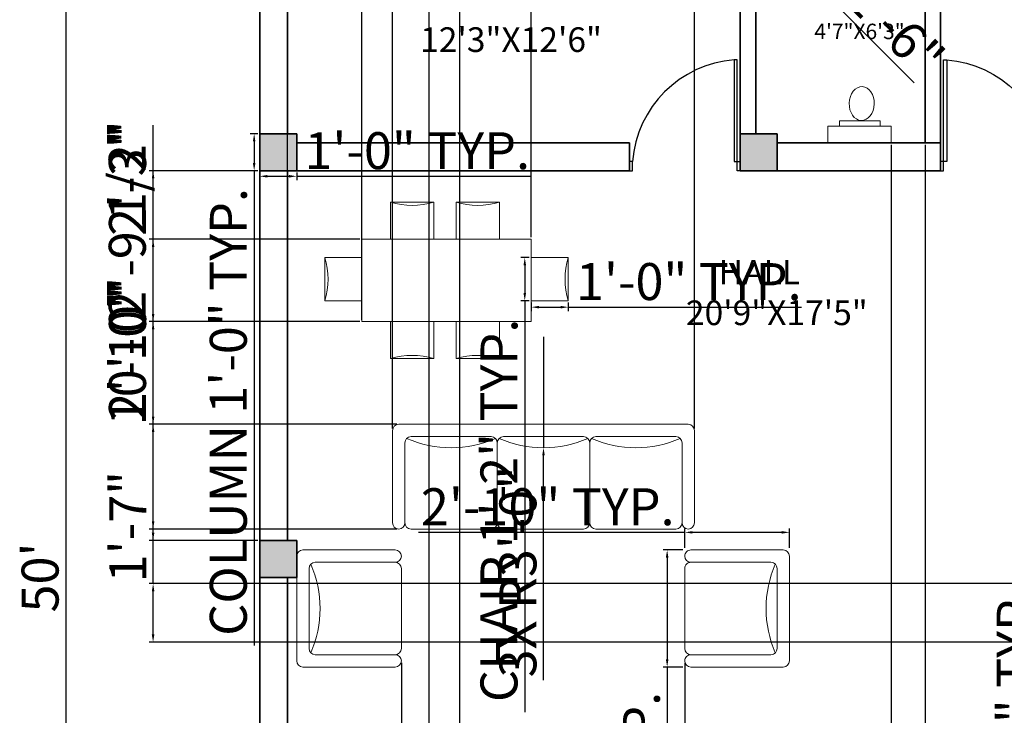
# Model space of a CAD drawing. Units: inches. Extents: x 2430 to 3058, y 1630 to 2396.
# Tile 2 of 4: x 2558 to 2878, y 1945 to 2171. Entities that reach past the tile are written whole.
import ezdxf

# ---------------------------------------------------------------- set-up
doc = ezdxf.new("R2010")
doc.units = ezdxf.units.IN
for name, color, linetype, lineweight in [('A-ANNO-DIMS', 7, 'Continuous', 18), ('A-AREA-IDEN', 131, 'Continuous', 18), ('A-COLS', 7, 'Continuous', 35), ('A-COLS-PATT', 1, 'Continuous', 13), ('A-DOOR', 40, 'Continuous', 25), ('A-FLOR-FIXT', 2, 'Continuous', 18), ('A-WALL', 7, 'Continuous', 35)]:
    doc.layers.add(name, color=color, linetype=linetype, lineweight=lineweight)
doc.layers.add('A-FURN', color=33, linetype='Continuous', lineweight=18, true_color=0xb0a07d)
doc.styles.get("Standard").update_dxf_attribs({"font": 'arial.ttf'})
doc.dimstyles.new('ISO-25', dxfattribs={"dimtxt": 12, "dimasz": 2.5, "dimexe": 1.25, "dimexo": 0.625, "dimtad": 1, "dimdec": 0, "dimlunit": 3, "dimtxsty": 'Standard', "dimcen": 2.5, "dimadec": 0, "dimazin": 0, "dimtfac": 1, "dimtdec": 0, "dimtmove": 0, "dimatfit": 3, "dimfxl": 1, "dimarcsym": 0})

# ---------------------------------------------------------------- blocks, each defined once
blk = doc.blocks.new('*D2')
at = {"layer": 'A-ANNO-DIMS', "color": 0, "lineweight": -2, "transparency": 16777216}
for p, q in [((2635.37, 2289.88), (2571.77, 2289.88)), ((2573.02, 2287.38), (2573.02, 1692.38)), ((2635.37, 1689.88), (2571.77, 1689.88))]:
    blk.add_line(p, q, dxfattribs=at)
at = {"layer": 'A-ANNO-DIMS', "color": 0, "transparency": 16777216}
for points in [[(2572.61, 2287.38), (2573.44, 2287.38), (2573.02, 2289.88)], [(2572.61, 1692.38), (2573.44, 1692.38), (2573.02, 1689.88)]]:
    blk.add_solid(points, dxfattribs=at)
at = {"layer": 'Defpoints', "color": 0, "transparency": 16777216}
for p in [(2636, 2289.88), (2573.02, 1689.88), (2636, 1689.88)]:
    blk.add_point(p, dxfattribs=at)
at = {"layer": 'A-ANNO-DIMS', "color": 0, "transparency": 16777216, "insert": (2566.27, 1989.88), "char_height": 12, "attachment_point": 5, "rotation": 90}
blk.add_mtext("50'", dxfattribs=at)
blk = doc.blocks.new('WC')
for points in [[(0, 18.29), (20.63, 18.29), (20.63, 12.83), (0, 12.83)], [(3.58, 12.83), (16.78, 12.83), (16.78, 11.1), (3.58, 11.1)]]:
    blk.add_lwpolyline(points, close=True)
blk.add_ellipse((9.59, 5.49), major_axis=(0.18, 5.49), ratio=0.738535)
blk = doc.blocks.new('ARMCHAIR')
for p, q in [((0, 2), (0, 36)), ((2, 38), (32, 38)), ((34, 36), (34, 36)), ((4, 6), (4, 32)), ((6, 34), (32, 34)), ((34, 32), (34, 6)), ((32, 4), (6, 4)), ((32, 0), (2, 0)), ((34, 2), (34, 2))]:
    blk.add_line(p, q)
for centre, radius, start, end in [((2, 36), 2, 90, 180), ((32, 36), 2, 0, 90), ((32, 36), 2, 270, 0), ((6, 32), 2, 90, 180), ((-28.4, 19), 36, 336.3971, 23.6029), ((32, 32), 2, 0, 90), ((6, 6), 2, 180, 270), ((32, 6), 2, 270, 0), ((32, 2), 2, 0, 90), ((2, 2), 2, 180, 270), ((32, 2), 2, 270, 0)]:
    blk.add_arc(centre, radius, start, end)
blk = doc.blocks.new('DOOR-36')
for p, q in [((35, 36), (34, 36)), ((34, 36), (34, 3)), ((35, 0), (35, 36)), ((1, 3), (0, 3)), ((0, 0), (1, 0)), ((1, 0), (1, 3)), ((34, 3), (36, 3)), ((36, 0), (35, 0))]:
    blk.add_line(p, q)
blk.add_arc((36.88, 0.12), 36, 94.5954, 175.4046)
blk = doc.blocks.new('CHAIR-DINING')
for p, q in [((0, 0), (0, 12)), ((0, 12), (14, 12)), ((14, 12), (14, 0))]:
    blk.add_line(p, q)
blk.add_arc((7, 34.96), 24, 253.0422, 286.9578)
blk = doc.blocks.new('COL-12x12-EDGE')
for p, q in [((12, 12), (0, 12)), ((0, 12), (0, 0)), ((0, 0), (12, 0))]:
    blk.add_line(p, q)
blk = doc.blocks.new('COL-12x12')
for p, q in [((12, 12), (0, 12)), ((0, 12), (0, 0)), ((12, 0), (12, 12)), ((0, 0), (12, 0))]:
    blk.add_line(p, q)
blk = doc.blocks.new('*D13')
at = {"layer": 'A-ANNO-DIMS', "color": 0, "lineweight": -2, "transparency": 16777216}
for p, q in [((2635.37, 2133.88), (2632.95, 2133.88)), ((2634.2, 2131.38), (2634.2, 2124.38)), ((2635.37, 2121.88), (2632.95, 2121.88)), ((2634.2, 2121.88), (2634.2, 1967.82))]:
    blk.add_line(p, q, dxfattribs=at)
at = {"layer": 'A-ANNO-DIMS', "color": 0, "transparency": 16777216}
for points in [[(2633.78, 2131.38), (2634.61, 2131.38), (2634.2, 2133.88)], [(2633.78, 2124.38), (2634.61, 2124.38), (2634.2, 2121.88)]]:
    blk.add_solid(points, dxfattribs=at)
at = {"layer": 'Defpoints', "color": 0, "transparency": 16777216}
for p in [(2636, 2133.88), (2634.2, 2121.88), (2636, 2121.88)]:
    blk.add_point(p, dxfattribs=at)
at = {"layer": 'A-ANNO-DIMS', "color": 0, "transparency": 16777216, "insert": (2627.36, 2043.6), "char_height": 12, "attachment_point": 5, "rotation": 90}
blk.add_mtext('COLUMN 1\'-0" TYP.', dxfattribs=at)
blk = doc.blocks.new('*D14')
at = {"layer": 'A-ANNO-DIMS', "color": 0, "lineweight": -2, "transparency": 16777216}
for p, q in [((2636, 2121.25), (2636, 2118.83)), ((2638.5, 2120.08), (2645.5, 2120.08)), ((2648, 2121.25), (2648, 2118.83)), ((2648, 2120.08), (2723.76, 2120.08))]:
    blk.add_line(p, q, dxfattribs=at)
at = {"layer": 'A-ANNO-DIMS', "color": 0, "transparency": 16777216}
for points in [[(2638.5, 2120.49), (2638.5, 2119.66), (2636, 2120.08)], [(2645.5, 2120.49), (2645.5, 2119.66), (2648, 2120.08)]]:
    blk.add_solid(points, dxfattribs=at)
at = {"layer": 'Defpoints', "color": 0, "transparency": 16777216}
for p in [(2636, 2121.88), (2648, 2121.88), (2648, 2120.08)]:
    blk.add_point(p, dxfattribs=at)
at = {"layer": 'A-ANNO-DIMS', "color": 0, "transparency": 16777216, "insert": (2687.13, 2126.83), "char_height": 12, "attachment_point": 5}
blk.add_mtext('1\'-0" TYP.', dxfattribs=at)
blk = doc.blocks.new('*D19')
at = {"layer": 'A-ANNO-DIMS', "color": 0, "lineweight": -2, "transparency": 16777216}
for p, q in [((2894.37, 2028.88), (2888.35, 2028.88)), ((2889.6, 2026.38), (2889.6, 1995.38)), ((2894.37, 1992.88), (2888.35, 1992.88)), ((2889.6, 1992.88), (2889.6, 1861.63))]:
    blk.add_line(p, q, dxfattribs=at)
at = {"layer": 'A-ANNO-DIMS', "color": 0, "transparency": 16777216}
for points in [[(2889.18, 2026.38), (2890.01, 2026.38), (2889.6, 2028.88)], [(2889.18, 1995.38), (2890.01, 1995.38), (2889.6, 1992.88)]]:
    blk.add_solid(points, dxfattribs=at)
at = {"layer": 'Defpoints', "color": 0, "transparency": 16777216}
for p in [(2895, 2028.88), (2889.6, 1992.88), (2895, 1992.88)]:
    blk.add_point(p, dxfattribs=at)
at = {"layer": 'A-ANNO-DIMS', "color": 0, "transparency": 16777216, "insert": (2882.76, 1926), "char_height": 12, "attachment_point": 5, "rotation": 90}
blk.add_mtext('DOOR 3\'-0" TYP.', dxfattribs=at)
blk = doc.blocks.new('*D23')
at = {"layer": 'A-ANNO-DIMS', "color": 0, "lineweight": -2, "transparency": 16777216}
for p, q in [((2723.51, 2093.7), (2720.79, 2093.7)), ((2722.04, 2091.2), (2722.04, 2082.2)), ((2723.51, 2079.7), (2720.79, 2079.7)), ((2722.04, 2079.7), (2722.04, 1946.13))]:
    blk.add_line(p, q, dxfattribs=at)
at = {"layer": 'A-ANNO-DIMS', "color": 0, "transparency": 16777216}
for points in [[(2721.62, 2091.2), (2722.45, 2091.2), (2722.04, 2093.7)], [(2721.62, 2082.2), (2722.45, 2082.2), (2722.04, 2079.7)]]:
    blk.add_solid(points, dxfattribs=at)
at = {"layer": 'Defpoints', "color": 0, "transparency": 16777216}
for p in [(2724.14, 2093.7), (2722.04, 2079.7), (2724.14, 2079.7)]:
    blk.add_point(p, dxfattribs=at)
at = {"layer": 'A-ANNO-DIMS', "color": 0, "transparency": 16777216, "insert": (2715.21, 2011.66), "char_height": 12, "attachment_point": 5, "rotation": 90}
blk.add_mtext('CHAIR 1\'-2" TYP.', dxfattribs=at)
blk = doc.blocks.new('*D24')
at = {"layer": 'A-ANNO-DIMS', "color": 0, "lineweight": -2, "transparency": 16777216}
for p, q in [((2724.14, 2079.08), (2724.14, 2076.35)), ((2726.64, 2077.6), (2733.64, 2077.6)), ((2736.14, 2079.08), (2736.14, 2076.35)), ((2736.14, 2077.6), (2811.9, 2077.6))]:
    blk.add_line(p, q, dxfattribs=at)
at = {"layer": 'A-ANNO-DIMS', "color": 0, "transparency": 16777216}
for points in [[(2726.64, 2078.02), (2726.64, 2077.18), (2724.14, 2077.6)], [(2733.64, 2078.02), (2733.64, 2077.18), (2736.14, 2077.6)]]:
    blk.add_solid(points, dxfattribs=at)
at = {"layer": 'Defpoints', "color": 0, "transparency": 16777216}
for p in [(2724.14, 2079.7), (2736.14, 2079.7), (2736.14, 2077.6)]:
    blk.add_point(p, dxfattribs=at)
at = {"layer": 'A-ANNO-DIMS', "color": 0, "transparency": 16777216, "insert": (2775.27, 2084.35), "char_height": 12, "attachment_point": 5}
blk.add_mtext('1\'-0" TYP.', dxfattribs=at)
blk = doc.blocks.new('*D25')
at = {"layer": 'A-ANNO-DIMS', "color": 0, "lineweight": -2, "transparency": 16777216}
for p, q in [((2773.33, 1998.82), (2767, 1998.82)), ((2768.25, 1996.32), (2768.25, 1963.32)), ((2773.33, 1960.82), (2767, 1960.82)), ((2768.25, 1960.82), (2768.25, 1789.16))]:
    blk.add_line(p, q, dxfattribs=at)
at = {"layer": 'A-ANNO-DIMS', "color": 0, "transparency": 16777216}
for points in [[(2767.83, 1996.32), (2768.67, 1996.32), (2768.25, 1998.82)], [(2767.83, 1963.32), (2768.67, 1963.32), (2768.25, 1960.82)]]:
    blk.add_solid(points, dxfattribs=at)
at = {"layer": 'Defpoints', "color": 0, "transparency": 16777216}
for p in [(2773.95, 1998.82), (2768.25, 1960.82), (2773.95, 1960.82)]:
    blk.add_point(p, dxfattribs=at)
at = {"layer": 'A-ANNO-DIMS', "color": 0, "transparency": 16777216, "insert": (2761.42, 1873.74), "char_height": 12, "attachment_point": 5, "rotation": 90}
blk.add_mtext('ARMCHAIR 3\'-2" TYP.', dxfattribs=at)
blk = doc.blocks.new('*D26')
at = {"layer": 'A-ANNO-DIMS', "color": 0, "lineweight": -2, "transparency": 16777216}
for p, q in [((2773.95, 2004.52), (2687.53, 2004.52)), ((2773.95, 1999.45), (2773.95, 2005.77)), ((2805.45, 2004.52), (2776.45, 2004.52)), ((2807.95, 1999.45), (2807.95, 2005.77))]:
    blk.add_line(p, q, dxfattribs=at)
at = {"layer": 'A-ANNO-DIMS', "color": 0, "transparency": 16777216}
for points in [[(2776.45, 2004.94), (2776.45, 2004.11), (2773.95, 2004.52)], [(2805.45, 2004.94), (2805.45, 2004.11), (2807.95, 2004.52)]]:
    blk.add_solid(points, dxfattribs=at)
at = {"layer": 'Defpoints', "color": 0, "transparency": 16777216}
for p in [(2773.95, 2004.52), (2773.95, 1998.82), (2807.95, 1998.82)]:
    blk.add_point(p, dxfattribs=at)
at = {"layer": 'A-ANNO-DIMS', "color": 0, "transparency": 16777216, "insert": (2729.49, 2011.28), "char_height": 12, "attachment_point": 5}
blk.add_mtext('2\'-10" TYP.', dxfattribs=at)
blk = doc.blocks.new('*D44')
at = {"layer": 'A-ANNO-DIMS', "color": 0, "lineweight": -2, "transparency": 16777216}
for p, q in [((2691, 1913.5), (2691, 2325.73)), ((2693.5, 2324.48), (2698.5, 2324.48)), ((2701, 1913.5), (2701, 2325.73)), ((2701, 2324.48), (2745.97, 2324.48))]:
    blk.add_line(p, q, dxfattribs=at)
at = {"layer": 'A-ANNO-DIMS', "color": 0, "transparency": 16777216}
for points in [[(2693.5, 2324.89), (2693.5, 2324.06), (2691, 2324.48)], [(2698.5, 2324.89), (2698.5, 2324.06), (2701, 2324.48)]]:
    blk.add_solid(points, dxfattribs=at)
at = {"layer": 'Defpoints', "color": 0, "transparency": 16777216}
for p in [(2701, 2324.48), (2691, 1912.88), (2701, 1912.88)]:
    blk.add_point(p, dxfattribs=at)
at = {"layer": 'A-ANNO-DIMS', "color": 0, "transparency": 16777216, "insert": (2724.73, 2331.23), "char_height": 12, "attachment_point": 5}
blk.add_mtext('0\'-10"', dxfattribs=at)
blk = doc.blocks.new('*D49')
at = {"layer": 'A-ANNO-DIMS', "color": 0, "lineweight": -2, "transparency": 16777216}
for p, q in [((2840.99, 2130.25), (2840.99, 1630.03)), ((2852, 2130.25), (2852, 1630.03)), ((2843.49, 1631.28), (2849.5, 1631.28)), ((2852, 1631.28), (2896.97, 1631.28))]:
    blk.add_line(p, q, dxfattribs=at)
at = {"layer": 'A-ANNO-DIMS', "color": 0, "transparency": 16777216}
for points in [[(2843.49, 1631.69), (2843.49, 1630.86), (2840.99, 1631.28)], [(2849.5, 1631.69), (2849.5, 1630.86), (2852, 1631.28)]]:
    blk.add_solid(points, dxfattribs=at)
at = {"layer": 'Defpoints', "color": 0, "transparency": 16777216}
for p in [(2840.99, 2130.88), (2852, 2130.88), (2852, 1631.28)]:
    blk.add_point(p, dxfattribs=at)
at = {"layer": 'A-ANNO-DIMS', "color": 0, "transparency": 16777216, "insert": (2875.73, 1638.03), "char_height": 12, "attachment_point": 5}
blk.add_mtext('0\'-11"', dxfattribs=at)
blk = doc.blocks.new('*D51')
at = {"layer": 'A-ANNO-DIMS', "color": 0, "lineweight": -2, "transparency": 16777216}
for p, q in [((2601.4, 1987.88), (2601.4, 2022.4)), ((2899.37, 1987.88), (2600.15, 1987.88)), ((2601.4, 1971.38), (2601.4, 1985.38)), ((2899.37, 1968.88), (2600.15, 1968.88))]:
    blk.add_line(p, q, dxfattribs=at)
at = {"layer": 'A-ANNO-DIMS', "color": 0, "transparency": 16777216}
for points in [[(2600.98, 1985.38), (2601.81, 1985.38), (2601.4, 1987.88)], [(2600.98, 1971.38), (2601.81, 1971.38), (2601.4, 1968.88)]]:
    blk.add_solid(points, dxfattribs=at)
at = {"layer": 'Defpoints', "color": 0, "transparency": 16777216}
for p in [(2601.4, 1987.88), (2900, 1987.88), (2900, 1968.88)]:
    blk.add_point(p, dxfattribs=at)
at = {"layer": 'A-ANNO-DIMS', "color": 0, "transparency": 16777216, "insert": (2594.75, 2006.39), "char_height": 12, "attachment_point": 5, "rotation": 90}
blk.add_mtext('1\'-7"', dxfattribs=at)
blk = doc.blocks.new('*D58')
at = {"layer": 'A-ANNO-DIMS', "color": 0, "lineweight": -2, "transparency": 16777216}
for p, q in [((2669.13, 2100.28), (2669.13, 2325.73)), ((2671.63, 2324.48), (2721.64, 2324.48)), ((2724.14, 2100.28), (2724.14, 2325.73))]:
    blk.add_line(p, q, dxfattribs=at)
at = {"layer": 'A-ANNO-DIMS', "color": 0, "transparency": 16777216}
for points in [[(2671.63, 2324.89), (2671.63, 2324.06), (2669.13, 2324.48)], [(2721.64, 2324.89), (2721.64, 2324.06), (2724.14, 2324.48)]]:
    blk.add_solid(points, dxfattribs=at)
at = {"layer": 'Defpoints', "color": 0, "transparency": 16777216}
for p in [(2724.14, 2324.48), (2669.13, 2099.65), (2724.14, 2099.65)]:
    blk.add_point(p, dxfattribs=at)
at = {"layer": 'A-ANNO-DIMS', "color": 0, "transparency": 16777216, "insert": (2696.63, 2331.1), "char_height": 12, "attachment_point": 5}
blk.add_mtext('4\'-7"', dxfattribs=at)
blk = doc.blocks.new('*D59')
at = {"layer": 'A-ANNO-DIMS', "color": 0, "lineweight": -2, "transparency": 16777216}
for p, q in [((2601.4, 2099.65), (2601.4, 2135.51)), ((2668.5, 2099.65), (2600.15, 2099.65)), ((2601.4, 2075.4), (2601.4, 2097.15)), ((2668.5, 2072.9), (2600.15, 2072.9))]:
    blk.add_line(p, q, dxfattribs=at)
at = {"layer": 'A-ANNO-DIMS', "color": 0, "transparency": 16777216}
for points in [[(2600.98, 2097.15), (2601.81, 2097.15), (2601.4, 2099.65)], [(2600.98, 2075.4), (2601.81, 2075.4), (2601.4, 2072.9)]]:
    blk.add_solid(points, dxfattribs=at)
at = {"layer": 'Defpoints', "color": 0, "transparency": 16777216}
for p in [(2601.4, 2099.65), (2669.13, 2099.65), (2669.13, 2072.9)]:
    blk.add_point(p, dxfattribs=at)
at = {"layer": 'A-ANNO-DIMS', "color": 0, "transparency": 16777216, "insert": (2594.64, 2118.83), "char_height": 12, "attachment_point": 5, "rotation": 90}
blk.add_mtext('2\'-3"', dxfattribs=at)
blk = doc.blocks.new('*D60')
at = {"layer": 'A-ANNO-DIMS', "color": 0, "lineweight": -2, "transparency": 16777216}
for p, q in [((2679.11, 2038.23), (2679.11, 2325.73)), ((2681.61, 2324.48), (2774.61, 2324.48)), ((2777.11, 2038.23), (2777.11, 2325.73))]:
    blk.add_line(p, q, dxfattribs=at)
at = {"layer": 'A-ANNO-DIMS', "color": 0, "transparency": 16777216}
for points in [[(2681.61, 2324.89), (2681.61, 2324.06), (2679.11, 2324.48)], [(2774.61, 2324.89), (2774.61, 2324.06), (2777.11, 2324.48)]]:
    blk.add_solid(points, dxfattribs=at)
at = {"layer": 'Defpoints', "color": 0, "transparency": 16777216}
for p in [(2777.11, 2324.48), (2679.11, 2037.6), (2777.11, 2037.6)]:
    blk.add_point(p, dxfattribs=at)
at = {"layer": 'A-ANNO-DIMS', "color": 0, "transparency": 16777216, "insert": (2728.11, 2331.23), "char_height": 12, "attachment_point": 5}
blk.add_mtext('8\'-2"', dxfattribs=at)
blk = doc.blocks.new('*D61')
at = {"layer": 'A-ANNO-DIMS', "color": 0, "lineweight": -2, "transparency": 16777216}
for p, q in [((2601.4, 2039.6), (2601.4, 2084.78)), ((2680.49, 2039.6), (2600.15, 2039.6)), ((2601.4, 2008.1), (2601.4, 2037.1)), ((2680.49, 2005.6), (2600.15, 2005.6))]:
    blk.add_line(p, q, dxfattribs=at)
at = {"layer": 'A-ANNO-DIMS', "color": 0, "transparency": 16777216}
for points in [[(2600.98, 2037.1), (2601.81, 2037.1), (2601.4, 2039.6)], [(2600.98, 2008.1), (2601.81, 2008.1), (2601.4, 2005.6)]]:
    blk.add_solid(points, dxfattribs=at)
at = {"layer": 'Defpoints', "color": 0, "transparency": 16777216}
for p in [(2601.4, 2039.6), (2681.11, 2039.6), (2681.11, 2005.6)]:
    blk.add_point(p, dxfattribs=at)
at = {"layer": 'A-ANNO-DIMS', "color": 0, "transparency": 16777216, "insert": (2594.64, 2063.44), "char_height": 12, "attachment_point": 5, "rotation": 90}
blk.add_mtext('2\'-10"', dxfattribs=at)
blk = doc.blocks.new('*D62')
at = {"layer": 'A-ANNO-DIMS', "color": 0, "lineweight": -2, "transparency": 16777216}
for p, q in [((2635.37, 2121.88), (2600.15, 2121.88)), ((2601.4, 2004.38), (2601.4, 2119.38)), ((2635.37, 2001.88), (2600.15, 2001.88))]:
    blk.add_line(p, q, dxfattribs=at)
at = {"layer": 'A-ANNO-DIMS', "color": 0, "transparency": 16777216}
for points in [[(2600.98, 2119.38), (2601.81, 2119.38), (2601.4, 2121.88)], [(2600.98, 2004.38), (2601.81, 2004.38), (2601.4, 2001.88)]]:
    blk.add_solid(points, dxfattribs=at)
at = {"layer": 'Defpoints', "color": 0, "transparency": 16777216}
for p in [(2601.4, 2121.88), (2636, 2121.88), (2636, 2001.88)]:
    blk.add_point(p, dxfattribs=at)
at = {"layer": 'A-ANNO-DIMS', "color": 0, "transparency": 16777216, "insert": (2594.64, 2061.88), "char_height": 12, "attachment_point": 5, "rotation": 90}
blk.add_mtext('10\'-0"', dxfattribs=at)
blk = doc.blocks.new('*D63')
at = {"layer": 'A-ANNO-DIMS', "color": 0, "lineweight": -2, "transparency": 16777216}
for p, q in [((2645, 2002.5), (2645, 2325.73)), ((2647.5, 2324.48), (2666.63, 2324.48)), ((2669.13, 2073.52), (2669.13, 2325.73)), ((2669.13, 2324.48), (2704.98, 2324.48))]:
    blk.add_line(p, q, dxfattribs=at)
at = {"layer": 'A-ANNO-DIMS', "color": 0, "transparency": 16777216}
for points in [[(2647.5, 2324.89), (2647.5, 2324.06), (2645, 2324.48)], [(2666.63, 2324.89), (2666.63, 2324.06), (2669.13, 2324.48)]]:
    blk.add_solid(points, dxfattribs=at)
at = {"layer": 'Defpoints', "color": 0, "transparency": 16777216}
for p in [(2669.13, 2324.48), (2669.13, 2072.9), (2645, 2001.88)]:
    blk.add_point(p, dxfattribs=at)
at = {"layer": 'A-ANNO-DIMS', "color": 0, "transparency": 16777216, "insert": (2688.3, 2331.23), "char_height": 12, "attachment_point": 5}
blk.add_mtext('2\'-0"', dxfattribs=at)
blk = doc.blocks.new('*D64')
at = {"layer": 'A-ANNO-DIMS', "color": 0, "lineweight": -2, "transparency": 16777216}
for p, q in [((2601.4, 2072.9), (2601.4, 2136.71)), ((2668.5, 2072.9), (2600.15, 2072.9)), ((2601.4, 2042.1), (2601.4, 2070.4)), ((2680.49, 2039.6), (2600.15, 2039.6))]:
    blk.add_line(p, q, dxfattribs=at)
at = {"layer": 'A-ANNO-DIMS', "color": 0, "transparency": 16777216}
for points in [[(2600.98, 2070.4), (2601.81, 2070.4), (2601.4, 2072.9)], [(2600.98, 2042.1), (2601.81, 2042.1), (2601.4, 2039.6)]]:
    blk.add_solid(points, dxfattribs=at)
at = {"layer": 'Defpoints', "color": 0, "transparency": 16777216}
for p in [(2601.4, 2072.9), (2669.13, 2072.9), (2681.11, 2039.6)]:
    blk.add_point(p, dxfattribs=at)
at = {"layer": 'A-ANNO-DIMS', "color": 0, "transparency": 16777216, "insert": (2594.57, 2106.05), "char_height": 12, "attachment_point": 5, "rotation": 90}
blk.add_mtext('2\'-9 1/2"', dxfattribs=at)
blk = doc.blocks.new('*D65')
at = {"layer": 'A-ANNO-DIMS', "color": 0, "lineweight": -2, "transparency": 16777216}
for p, q in [((2682, 1962.2), (2682, 1630.03)), ((2773.95, 1962.2), (2773.95, 1630.03)), ((2684.5, 1631.28), (2771.45, 1631.28))]:
    blk.add_line(p, q, dxfattribs=at)
at = {"layer": 'A-ANNO-DIMS', "color": 0, "transparency": 16777216}
for points in [[(2684.5, 1631.69), (2684.5, 1630.86), (2682, 1631.28)], [(2771.45, 1631.69), (2771.45, 1630.86), (2773.95, 1631.28)]]:
    blk.add_solid(points, dxfattribs=at)
at = {"layer": 'Defpoints', "color": 0, "transparency": 16777216}
for p in [(2682, 1962.82), (2773.95, 1962.82), (2773.95, 1631.28)]:
    blk.add_point(p, dxfattribs=at)
at = {"layer": 'A-ANNO-DIMS', "color": 0, "transparency": 16777216, "insert": (2727.97, 1638.03), "char_height": 12, "attachment_point": 5}
blk.add_mtext('7\'-8"', dxfattribs=at)
blk = doc.blocks.new('*D67')
at = {"layer": 'A-ANNO-DIMS', "color": 0, "lineweight": -2, "transparency": 16777216}
for p, q in [((2728.11, 2068), (2728.11, 2032)), ((2728.11, 1956.59), (2728.11, 2029.5))]:
    blk.add_line(p, q, dxfattribs=at)
at = {"layer": 'A-ANNO-DIMS', "color": 0, "transparency": 16777216}
blk.add_solid([(2727.7, 2029.5), (2728.53, 2029.5), (2728.11, 2032)], dxfattribs=at)
at = {"layer": 'Defpoints', "color": 0, "transparency": 16777216}
for p in [(2728.11, 2068), (2728.11, 2032)]:
    blk.add_point(p, dxfattribs=at)
at = {"layer": 'A-ANNO-DIMS', "color": 0, "transparency": 16777216, "insert": (2721.36, 1991.8), "char_height": 12, "attachment_point": 5, "rotation": 89.9995}
blk.add_mtext('3X R3\'-0"', dxfattribs=at)
blk = doc.blocks.new('*D68')
at = {"layer": 'A-ANNO-DIMS', "color": 0, "lineweight": -2, "transparency": 16777216}
for p, q in [((2792.13, 2206.74), (2813.35, 2185.53)), ((2848.44, 2150.43), (2815.11, 2183.76))]:
    blk.add_line(p, q, dxfattribs=at)
at = {"layer": 'A-ANNO-DIMS', "color": 0, "transparency": 16777216}
blk.add_solid([(2815.41, 2184.05), (2814.82, 2183.47), (2813.35, 2185.53)], dxfattribs=at)
at = {"layer": 'Defpoints', "color": 0, "transparency": 16777216}
for p in [(2792.13, 2206.74), (2813.35, 2185.53)]:
    blk.add_point(p, dxfattribs=at)
at = {"layer": 'A-ANNO-DIMS', "color": 0, "transparency": 16777216, "insert": (2837.44, 2170.99), "char_height": 12, "attachment_point": 5, "rotation": 315.0012}
blk.add_mtext('R2\'-6"', dxfattribs=at)

msp = doc.modelspace()

# ---------------------------------------------------------------- hatches: boundary and pattern name
at = {"layer": 'A-COLS-PATT'}
h = msp.add_hatch(color=256, dxfattribs=at)
h.dxf.hatch_style = 1
h.paths.add_polyline_path([(2648, 2133.88), (2636, 2133.88), (2636, 2121.88), (2648, 2121.88)])
h = msp.add_hatch(color=256, dxfattribs=at)
h.dxf.hatch_style = 1
h.paths.add_polyline_path([(2804, 2133.88), (2792, 2133.88), (2792, 2121.88), (2804, 2121.88)])
h = msp.add_hatch(color=256, dxfattribs=at)
h.dxf.hatch_style = 1
h.paths.add_polyline_path([(2648, 1996.82), (2648, 2001.88), (2636, 2001.88), (2636, 1989.88), (2648, 1989.88)])

# ---------------------------------------------------------------- linework, layer by layer
at = {"layer": 'A-FURN'}
for p, q in [((2681.11, 2039.6), (2715.11, 2039.6)), ((2711.11, 2039.6), (2745.11, 2039.6)), ((2741.11, 2039.6), (2775.11, 2039.6)), ((2679.11, 2007.6), (2679.11, 2037.6)), ((2777.11, 2037.6), (2777.11, 2007.6)), ((2683.11, 2007.6), (2683.11, 2033.6)), ((2685.11, 2035.6), (2711.11, 2035.6)), ((2713.11, 2033.6), (2713.11, 2007.6)), ((2713.11, 2007.6), (2713.11, 2033.6)), ((2715.11, 2035.6), (2741.11, 2035.6)), ((2743.11, 2033.6), (2743.11, 2007.6)), ((2743.11, 2007.6), (2743.11, 2033.6)), ((2745.11, 2035.6), (2771.11, 2035.6)), ((2773.11, 2033.6), (2773.11, 2007.6)), ((2681.11, 2005.6), (2681.11, 2005.6)), ((2711.11, 2005.6), (2685.11, 2005.6)), ((2715.11, 2005.6), (2715.11, 2005.6)), ((2741.11, 2005.6), (2715.11, 2005.6)), ((2741.11, 2005.6), (2741.11, 2005.6)), ((2745.11, 2005.6), (2745.11, 2005.6)), ((2771.11, 2005.6), (2745.11, 2005.6)), ((2775.11, 2005.6), (2775.11, 2005.6))]:
    msp.add_line(p, q, dxfattribs=at)
msp.add_lwpolyline([(2669.13, 2099.65), (2724.14, 2099.65), (2724.14, 2072.9), (2669.13, 2072.9)], close=True, dxfattribs=at)
for centre, radius, start, end in [((2681.11, 2037.6), 2, 90, 180), ((2775.11, 2037.6), 2, 0, 90), ((2685.11, 2033.6), 2, 90, 180), ((2698.11, 2068), 36, 246.3971, 293.6029), ((2711.11, 2033.6), 2, 0, 90), ((2715.11, 2033.6), 2, 90, 180), ((2728.11, 2068), 36, 246.3971, 293.6029), ((2741.11, 2033.6), 2, 0, 90), ((2745.11, 2033.6), 2, 90, 180), ((2758.11, 2068), 36, 246.3971, 293.6029), ((2771.11, 2033.6), 2, 0, 90), ((2681.11, 2007.6), 2, 180, 270), ((2681.11, 2007.6), 2, 270, 0), ((2685.11, 2007.6), 2, 180, 270), ((2711.11, 2007.6), 2, 270, 0), ((2711.11, 2007.6), 2, 270, 0), ((2715.11, 2007.6), 2, 180, 270), ((2741.11, 2007.6), 2, 270, 0), ((2745.11, 2007.6), 2, 180, 270), ((2771.11, 2007.6), 2, 270, 0), ((2775.11, 2007.6), 2, 180, 270), ((2775.11, 2007.6), 2, 270, 0)]:
    msp.add_arc(centre, radius, start, end, dxfattribs=at)
at = {"layer": 'A-WALL'}
for p, q in [((2645, 2133.88), (2645, 2277.88)), ((2852, 2130.88), (2852, 2210.88)), ((2857, 2121.88), (2857, 2210.88)), ((2792, 2121.88), (2792, 2175.88)), ((2797, 2133.88), (2797, 2175.88)), ((2648, 2130.88), (2756, 2130.88)), ((2756, 2121.88), (2756, 2130.88)), ((2804, 2130.88), (2857, 2130.88)), ((2645, 2121.88), (2756, 2121.88)), ((2645, 2001.88), (2645, 2121.88)), ((2792, 2121.88), (2857, 2121.88)), ((2645, 1860.88), (2645, 1989.88))]:
    msp.add_line(p, q, dxfattribs=at)
msp.add_lwpolyline([(2636, 2289.88), (2996, 2289.88), (2996, 1689.88), (2636, 1689.88)], close=True, dxfattribs=at)

# ---------------------------------------------------------------- block references
at = {"layer": 'A-COLS'}
for name, p, rotation in [('COL-12x12', (2636, 2133.88), 270.0000000000065), ('COL-12x12-EDGE', (2804, 2133.88), 180), ('COL-12x12-EDGE', (2648, 2001.88), 180)]:
    msp.add_blockref(name, p, dxfattribs=dict(at, rotation=rotation))
at = {"layer": 'A-DOOR'}
msp.add_blockref('DOOR-36', (2756, 2121.88), dxfattribs=at)
at = {"layer": 'A-DOOR', "extrusion": (0, 0, -1), "zscale": -1}
msp.add_blockref('DOOR-36', (-2893, 2121.88), dxfattribs=at)
at = {"layer": 'A-FLOR-FIXT', "rotation": 180}
msp.add_blockref('WC', (2840.99, 2149.17), dxfattribs=at)
at = {"layer": 'A-FURN'}
for name, p in [('CHAIR-DINING', (2678.48, 2099.65)), ('CHAIR-DINING', (2699.78, 2099.65)), ('ARMCHAIR', (2648, 1960.82))]:
    msp.add_blockref(name, p, dxfattribs=at)
for name, p, rotation in [('CHAIR-DINING', (2669.13, 2079.7), 89.99999999999775), ('CHAIR-DINING', (2724.14, 2093.7), 270.0000000000022), ('CHAIR-DINING', (2692.48, 2072.9), 180), ('CHAIR-DINING', (2713.78, 2072.9), 180), ('ARMCHAIR', (2807.95, 1998.82), 180)]:
    msp.add_blockref(name, p, dxfattribs=dict(at, rotation=rotation))

# ---------------------------------------------------------------- texts
at = {"layer": 'A-AREA-IDEN'}
for tag, p, height in [('12\'3"X12\'6"', (2688.07, 2160.42), 8), ('4\'7"X6\'3"', (2816.03, 2164.59), 5), ('HALL', (2784.97, 2084.96), 8), ('20\'9"X17\'5"', (2774.34, 2071.78), 8)]:
    msp.add_attdef(tag, p, '', height=height, dxfattribs=at)

# ---------------------------------------------------------------- dimensions: what is measured, and where the dimension line sits
at = {"layer": 'A-ANNO-DIMS'}
for base, p1, p2, picture, middle in [((2669.13, 2324.48), (2645, 2001.88), (2669.13, 2072.9), '*D63', (2688.3, 2331.23)), ((2777.11, 2324.48), (2679.11, 2037.6), (2777.11, 2037.6), '*D60', (2728.11, 2331.23)), ((2701, 2324.48), (2691, 1912.88), (2701, 1912.88), '*D44', (2724.73, 2331.23)), ((2724.14, 2324.48), (2669.13, 2099.65), (2724.14, 2099.65), '*D58', (2696.63, 2331.1)), ((2852, 1631.28), (2840.99, 2130.88), (2852, 2130.88), '*D49', (2875.73, 1638.03)), ((2773.9503, 1631.2777), (2681.9954, 1962.8232), (2773.9503, 1962.8232), '*D65', (2727.9729, 1638.0296))]:
    dim = msp.add_linear_dim(base=base, p1=p1, p2=p2, dimstyle='ISO-25', override={"dimdec": 1, "dimlfac": 1, "dimrnd": 0, "dimzin": 1, "dimdsep": 46, "dimlunit": 4, "dimfrac": 2}, dxfattribs=at)
    dim.commit()
    dim.dimension.update_dxf_attribs({"geometry": picture, "text_midpoint": middle})
for base, p1, p2, override, picture, middle in [((2573.02, 1689.88), (2636, 2289.88), (2636, 1689.88), {"dimclrd": 0, "dimclre": 0, "dimclrt": 0}, '*D2', (2566.27, 1989.88)), ((2601.4, 2072.9), (2681.11, 2039.6), (2669.13, 2072.9), {"dimdec": 1, "dimlfac": 1, "dimrnd": 0, "dimzin": 1, "dimdsep": 46, "dimlunit": 4, "dimfrac": 2}, '*D64', (2594.57, 2106.05)), ((2601.3954, 2099.6539), (2669.1274, 2072.8964), (2669.1274, 2099.6539), {"dimdec": 1, "dimlfac": 1, "dimrnd": 0, "dimzin": 1, "dimdsep": 46, "dimlunit": 4, "dimfrac": 2}, '*D59', (2594.6395, 2118.8307)), ((2601.4, 2121.88), (2636, 2001.88), (2636, 2121.88), {"dimdec": 1, "dimlfac": 1, "dimrnd": 0, "dimzin": 1, "dimdsep": 46, "dimlunit": 4, "dimfrac": 2}, '*D62', (2594.64, 2061.88)), ((2601.4, 2039.6), (2681.11, 2005.6), (2681.11, 2039.6), {"dimdec": 1, "dimlfac": 1, "dimrnd": 0, "dimzin": 1, "dimdsep": 46, "dimlunit": 4, "dimfrac": 2}, '*D61', (2594.64, 2063.44)), ((2601.4, 1987.88), (2900, 1968.88), (2900, 1987.88), {"dimdec": 1, "dimlfac": 1, "dimrnd": 0, "dimzin": 1, "dimdsep": 46, "dimlunit": 4, "dimfrac": 2}, '*D51', (2594.75, 2006.39))]:
    dim = msp.add_linear_dim(base=base, p1=p1, p2=p2, angle=90, dimstyle='ISO-25', override=override, dxfattribs=at)
    dim.commit()
    dim.dimension.update_dxf_attribs({"geometry": picture, "text_midpoint": middle})
dim = msp.add_radius_dim(center=(2792.13, 2206.74), mpoint=(2813.35, 2185.53), dimstyle='ISO-25', override={"dimdec": 1, "dimlfac": 1, "dimrnd": 0, "dimzin": 1, "dimdsep": 46, "dimlunit": 4, "dimfrac": 2}, dxfattribs=at)
dim.commit()
dim.dimension.update_dxf_attribs({"geometry": '*D68', "text_midpoint": (2837.44, 2170.99)})
for base, p1, p2, angle, text, picture, middle in [((2648, 2120.08), (2636, 2121.88), (2648, 2121.88), 0, '<> TYP.', '*D14', (2687.13, 2126.83)), ((2634.2, 2121.88), (2636, 2133.88), (2636, 2121.88), 270, 'COLUMN <> TYP.', '*D13', (2627.36, 2043.6)), ((2736.14, 2077.6), (2724.14, 2079.7), (2736.14, 2079.7), 0, '<> TYP.', '*D24', (2775.27, 2084.35)), ((2722.04, 2079.7), (2724.14, 2093.7), (2724.14, 2079.7), 270, 'CHAIR <> TYP.', '*D23', (2715.21, 2011.66)), ((2773.95, 2004.52), (2807.95, 1998.82), (2773.95, 1998.82), 180, '<> TYP.', '*D26', (2729.49, 2011.28)), ((2889.6, 1992.88), (2895, 2028.88), (2895, 1992.88), 270, 'DOOR <> TYP.', '*D19', (2882.76, 1926)), ((2768.25, 1960.82), (2773.95, 1998.82), (2773.95, 1960.82), 270, 'ARMCHAIR <> TYP.', '*D25', (2761.42, 1873.74))]:
    dim = msp.add_linear_dim(base=base, p1=p1, p2=p2, angle=angle, text=text, dimstyle='ISO-25', override={"dimdec": 1, "dimlfac": 1, "dimrnd": 0, "dimzin": 1, "dimdsep": 46, "dimlunit": 4, "dimfrac": 2}, dxfattribs=at)
    dim.commit()
    dim.dimension.update_dxf_attribs({"geometry": picture, "text_midpoint": middle})
dim = msp.add_radius_dim(center=(2728.11, 2068), mpoint=(2728.11, 2032), text='3X <>', dimstyle='ISO-25', override={"dimdec": 1, "dimlfac": 1, "dimrnd": 0, "dimzin": 1, "dimdsep": 46, "dimlunit": 4, "dimfrac": 2}, dxfattribs=at)
dim.commit()
dim.dimension.update_dxf_attribs({"geometry": '*D67', "text_midpoint": (2721.36, 1991.8)})

doc.saveas('drawing.dxf')
